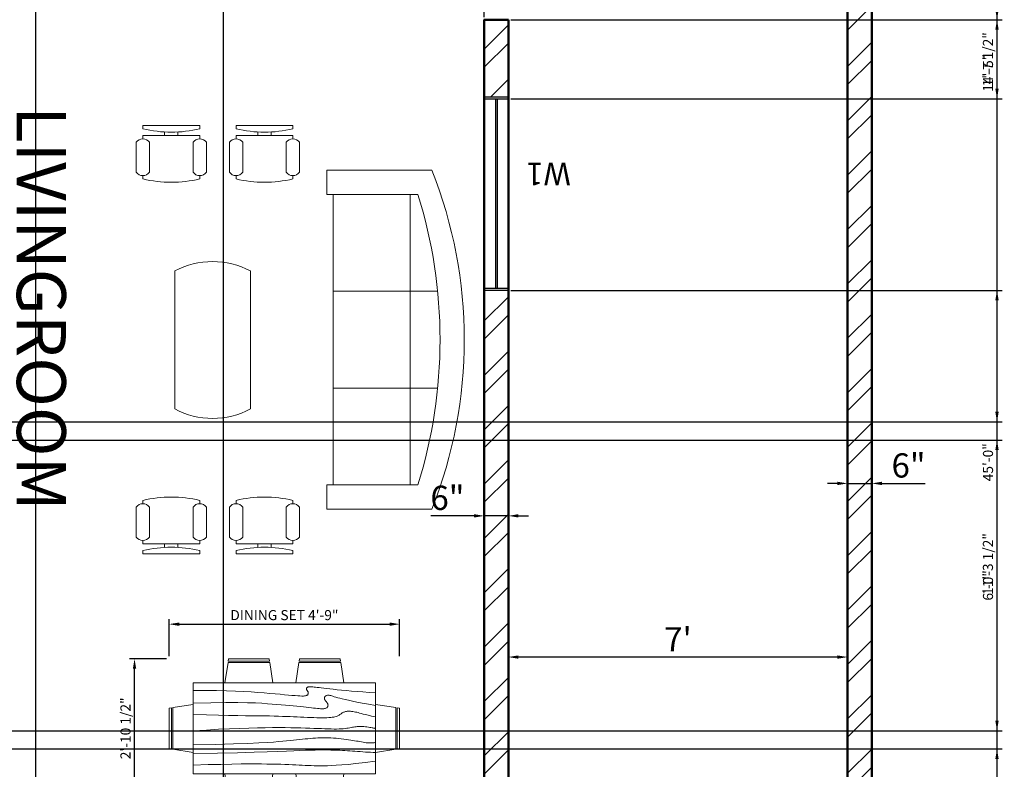
# Model space of a CAD drawing. Units: inches. Extents: x 244 to 2800, y 1060 to 1700.
# Tile 10 of 13: x 1781 to 2025, y 1287 to 1473. Entities that reach past the tile are written whole.
import ezdxf

# ---------------------------------------------------------------- set-up
doc = ezdxf.new("R2010")
doc.units = ezdxf.units.IN
for name, color, linetype, lineweight in [('A-ANNO-DIMS', 2, 'Continuous', 18), ('A-ANNO-TEXT', 1, 'Continuous', 18), ('A-FURN', 9, 'Continuous', 18), ('A-GLAZ', 3, 'Continuous', 25), ('A-WALL', 7, 'Continuous', 50), ('A-WALL-PATT', 8, 'Continuous', 13)]:
    doc.layers.add(name, color=color, linetype=linetype, lineweight=lineweight)
doc.styles.get("Standard").update_dxf_attribs({"font": 'arial.ttf'})
doc.dimstyles.new('ISO-25', dxfattribs={"dimtxt": 2.5, "dimasz": 2.5, "dimexe": 1.25, "dimexo": 0.625, "dimtad": 1, "dimlunit": 4, "dimtxsty": 'Standard', "dimcen": 2.5, "dimadec": 0, "dimazin": 0, "dimtfac": 1, "dimtmove": 0, "dimatfit": 3, "dimfxl": 1, "dimarcsym": 0})

# ---------------------------------------------------------------- blocks, each defined once
blk = doc.blocks.new('Chair - Desk')
for p, q in [((-8.5, 0), (-8.5, -1)), ((-8.5, 0), (8.5, 0)), ((8.5, 0), (8.5, -1)), ((-2, -3), (-2, -1.9355)), ((2, -1.9576), (2, -3)), ((-10.5, -5), (-10.5, -14)), ((-8.5, -3), (-8.5, -4)), ((-8.5, -3), (8.5, -3)), ((-6.5, -14), (-6.5, -5)), ((6.5, -5), (6.5, -14)), ((8.5, -3), (8.5, -4)), ((10.5, -14), (10.5, -5)), ((-8.5, -15), (-8.5, -16)), ((8.5, -15), (8.5, -16))]:
    blk.add_line(p, q)
for centre, radius, start, end in [((0, 34.625), 36.625, 256.5803, 283.4197), ((-8.5, -6.5), 2.5, 36.8699, 143.1301), ((8.5, -6.5), 2.5, 36.8699, 143.1301), ((-8.5, -12.5), 2.5, 216.8699, 323.1301), ((8.5, -12.5), 2.5, 216.8699, 323.1301), ((0, 19.625), 36.625, 256.5803, 283.4197)]:
    blk.add_arc(centre, radius, start, end)
blk = doc.blocks.new('Dining Set - 36 x 72 in.')
for p, q in [((-22, 27.5), (-22.1562, 26.50042)), ((-22, 27.5), (-6, 27.5)), ((-5.8437, 26.49966), (-6, 27.5)), ((6, 27.5), (5.8438, 26.50042)), ((6, 27.5), (22, 27.5)), ((22.1563, 26.49966), (22, 27.5)), ((-22.2343, 26.00059), (-23.4847, 17.99762)), ((-22.2304, 26), (-5.7608, 26)), ((-5.8416, 26.5), (-22.1534, 26.5)), ((-4.5152, 17.99762), (-5.7655, 25.99926)), ((5.7657, 26.00059), (4.5153, 17.99762)), ((5.7696, 26), (22.2392, 26)), ((22.1584, 26.5), (5.8466, 26.5)), ((23.4848, 17.99762), (22.2345, 25.99926)), ((36, 18), (-36, 18)), ((-36, 18), (-36, -18)), ((36, -18), (36, 18)), ((-45.5, 8), (-44.5004, 8.15617)), ((-45.5, 8), (-45.5, -8)), ((-44.5, -8.15843), (-44.5, 8.15338)), ((-44.0006, 8.23428), (-35.9976, 9.48474)), ((-44, 8.23041), (-44, -8.23915)), ((44.0006, 8.23428), (35.9976, 9.48474)), ((44, 8.23041), (44, -8.23915)), ((44.5, -8.15843), (44.5, 8.15338)), ((45.5, 8), (44.5005, 8.15617)), ((45.5, 8), (45.5, -8)), ((-44.4997, -8.15631), (-45.5, -8)), ((-35.9976, -9.48476), (-43.9993, -8.2345)), ((35.9976, -9.48476), (43.9993, -8.2345)), ((44.4997, -8.15631), (45.5, -8)), ((-36, -18), (36, -18)), ((-22.2343, -26.0006), (-23.4847, -17.99762)), ((-4.5152, -17.99762), (-5.7655, -25.99928)), ((5.7657, -26.0006), (4.5153, -17.99762)), ((23.4848, -17.99762), (22.2345, -25.99928)), ((-22.2304, -26), (-5.7608, -26)), ((-22, -27.5), (-22.1562, -26.50044)), ((-5.8416, -26.5), (-22.1534, -26.5)), ((-5.8437, -26.49967), (-6, -27.5)), ((5.7696, -26), (22.2392, -26)), ((6, -27.5), (5.8438, -26.50044)), ((22.1584, -26.5), (5.8466, -26.5)), ((22.1563, -26.49967), (22, -27.5)), ((-22, -27.5), (-6, -27.5)), ((6, -27.5), (22, -27.5))]:
    blk.add_line(p, q)
for points in [[(-36, 15), (-31.1772, 14.97754), (-26.8079, 14.91406), (-22.8538, 14.81543), (-19.276, 14.6875), (-16.0362, 14.53613), (-13.0957, 14.36718), (-10.4159, 14.18652), (-7.9583, 14), (-5.6904, 13.81315), (-3.6035, 13.63021), (-1.6954, 13.45508), (0.0365, 13.29166), (1.5945, 13.14388), (2.9811, 13.01562), (4.1988, 12.9108), (5.25, 12.83333), (6.1393, 12.78613), (6.8802, 12.76823), (7.4883, 12.77767), (7.9792, 12.8125), (8.3685, 12.87077), (8.6719, 12.95052), (8.9049, 13.0498), (9.0833, 13.16666), (9.2205, 13.29899), (9.3216, 13.44401), (9.3895, 13.59879), (9.4271, 13.76041), (9.4373, 13.92594), (9.4232, 14.09245), (9.3875, 14.257), (9.3333, 14.41666), (9.2638, 14.56917), (9.1836, 14.71484), (9.0975, 14.85465), (9.0104, 14.98958), (8.9272, 15.1206), (8.8529, 15.2487), (8.7922, 15.37483), (8.75, 15.5), (8.7305, 15.62467), (8.7344, 15.74739), (8.7617, 15.86621), (8.8125, 15.97916), (8.8867, 16.08431), (8.9844, 16.17968), (9.1055, 16.26334), (9.25, 16.33333), (9.4189, 16.38802), (9.6172, 16.42708), (9.8506, 16.45052), (10.125, 16.45833), (10.4463, 16.45052), (10.8203, 16.42708), (11.2529, 16.38802), (11.75, 16.33333), (12.3184, 16.26318), (12.9694, 16.17838), (13.7151, 16.07991), (14.5677, 15.96875), (15.5395, 15.84586), (16.6426, 15.71224), (17.8893, 15.56884), (19.2917, 15.41666), (20.859, 15.25667), (22.5879, 15.08984), (24.4721, 14.91715), (26.5052, 14.73958), (28.6809, 14.5581), (30.9929, 14.3737), (33.4347, 14.18733), (36, 14)], [(-36, 10), (-28.9766, 10.14274), (-23.1725, 10.20442), (-18.4241, 10.19775), (-14.5677, 10.13541), (-11.4399, 10.03011), (-8.877, 9.89453), (-6.7154, 9.74137), (-4.7917, 9.58333), (-2.9698, 9.43082), (-1.2246, 9.28515), (0.4415, 9.14534), (2.026, 9.01041), (3.5266, 8.87939), (4.9408, 8.7513), (6.266, 8.62516), (7.5, 8.5), (8.6411, 8.37549), (9.6914, 8.2539), (10.6538, 8.13818), (11.5312, 8.03125), (12.3267, 7.93603), (13.043, 7.85547), (13.6831, 7.79248), (14.25, 7.75), (14.7471, 7.7303), (15.1797, 7.73307), (15.5537, 7.75732), (15.875, 7.80208), (16.1494, 7.86637), (16.3828, 7.94922), (16.5811, 8.04964), (16.75, 8.16666), (16.8944, 8.29915), (17.0143, 8.44531), (17.1089, 8.60319), (17.1771, 8.77083), (17.218, 8.94629), (17.2305, 9.1276), (17.2137, 9.31282), (17.1667, 9.5), (17.0895, 9.6875), (16.987, 9.875), (16.8649, 10.0625), (16.7292, 10.25), (16.5856, 10.4375), (16.4401, 10.625), (16.2985, 10.8125), (16.1667, 11), (16.05, 11.18733), (15.9518, 11.3737), (15.8752, 11.5581), (15.8229, 11.73958), (15.798, 11.91715), (15.8034, 12.08984), (15.842, 12.25667), (15.9167, 12.41666), (16.0295, 12.56836), (16.1784, 12.70833), (16.3605, 12.83268), (16.5729, 12.9375), (16.8127, 13.01888), (17.0768, 13.07291), (17.3625, 13.0957), (17.6667, 13.08333), (17.9894, 13.03312), (18.3418, 12.94726), (18.7382, 12.82918), (19.1927, 12.68229), (19.7195, 12.51001), (20.3327, 12.31575), (21.0465, 12.10294), (21.875, 11.875), (22.8357, 11.63354), (23.959, 11.37304), (25.2786, 11.08618), (26.8282, 10.76562), (28.6414, 10.40405), (30.752, 9.99414), (33.1936, 9.52856), (36, 9)], [(-36, 5.5), (-30.7157, 5.3348), (-26.069, 5.20963), (-21.9946, 5.11767), (-18.4271, 5.05208), (-15.3009, 5.00602), (-12.5508, 4.97265), (-10.1112, 4.94515), (-7.9167, 4.91666), (-5.909, 4.88167), (-4.0586, 4.83984), (-2.3429, 4.79215), (-0.7396, 4.73958), (0.7739, 4.6831), (2.22, 4.6237), (3.6213, 4.56233), (5, 4.5), (6.373, 4.43782), (7.7344, 4.3776), (9.0723, 4.32129), (10.375, 4.27083), (11.6309, 4.22819), (12.8281, 4.19531), (13.9551, 4.17415), (15, 4.16666), (15.954, 4.17448), (16.819, 4.19791), (17.6001, 4.23698), (18.3021, 4.29166), (18.9299, 4.36198), (19.4883, 4.44791), (19.9823, 4.54948), (20.4167, 4.66666), (20.7969, 4.79899), (21.1302, 4.94401), (21.4245, 5.09879), (21.6875, 5.26041), (21.9271, 5.42594), (22.1511, 5.59245), (22.3672, 5.757), (22.5834, 5.91666), (22.8065, 6.06868), (23.0404, 6.21093), (23.2879, 6.34147), (23.5521, 6.45833), (23.8358, 6.55957), (24.142, 6.64323), (24.4735, 6.70735), (24.8334, 6.75), (25.2235, 6.76969), (25.642, 6.76692), (26.0858, 6.74267), (26.5521, 6.69791), (27.0379, 6.63362), (27.5404, 6.55078), (28.0565, 6.45036), (28.5834, 6.33333), (29.1242, 6.19987), (29.7071, 6.04687), (30.3661, 5.87044), (31.1354, 5.66666), (32.0493, 5.43164), (33.142, 5.16146), (34.4475, 4.85221), (36, 4.5)], [(-36, -1), (-30.7915, -0.6591), (-26.0195, -0.38216), (-21.6519, -0.16284), (-17.6563, 0.00521), (-14.0005, 0.12833), (-10.6523, 0.21289), (-7.5796, 0.26522), (-4.75, 0.29166), (-2.134, 0.29793), (0.2878, 0.28711), (2.5317, 0.26163), (4.6146, 0.22396), (6.5529, 0.17651), (8.3633, 0.12174), (10.0623, 0.06209), (11.6667, 0), (13.1899, -0.06201), (14.6341, -0.1211), (15.9982, -0.17432), (17.2813, -0.21875), (18.4823, -0.25147), (19.6003, -0.26953), (20.6343, -0.27002), (21.5834, -0.25), (22.4481, -0.20768), (23.2357, -0.14584), (23.9549, -0.06836), (24.6146, 0.02083), (25.2235, 0.11784), (25.7904, 0.21875), (26.3241, 0.31966), (26.8334, 0.41666), (27.3265, 0.50618), (27.8099, 0.58593), (28.2894, 0.65397), (28.7709, 0.70833), (29.2601, 0.74707), (29.763, 0.76823), (30.2855, 0.76985), (30.8334, 0.75), (31.4088, 0.70784), (31.9994, 0.64713), (32.589, 0.57275), (33.1615, 0.48958), (33.7008, 0.4025), (34.1908, 0.3164), (34.6153, 0.23616), (34.9584, 0.16666), (35.2099, 0.11165), (35.3848, 0.07031), (35.504, 0.04069), (35.5886, 0.02083), (35.6594, 0.00879), (35.7377, 0.0026), (35.8442, 0.00032), (36, 0)], [(-36, -6.5), (-27.1843, -6.31267), (-20.084, -6.1263), (-14.469, -5.9419), (-10.1094, -5.76042), (-6.7752, -5.58285), (-4.2363, -5.41016), (-2.2629, -5.24333), (-0.625, -5.08334), (0.8708, -4.93099), (2.2715, -4.78646), (3.5872, -4.64974), (4.8281, -4.52084), (6.0046, -4.39974), (7.127, -4.28646), (8.2053, -4.18099), (9.25, -4.08334), (10.2705, -3.99382), (11.2734, -3.91407), (12.2647, -3.84603), (13.25, -3.79167), (14.2354, -3.75293), (15.2266, -3.73177), (16.2295, -3.73015), (17.25, -3.75), (18.2912, -3.79248), (19.3451, -3.85547), (20.4009, -3.93604), (21.4479, -4.03125), (22.4754, -4.13819), (23.4727, -4.25391), (24.4289, -4.37549), (25.3334, -4.5), (26.1785, -4.62492), (26.9694, -4.74935), (27.7145, -4.87281), (28.4219, -4.99479), (29.1, -5.11483), (29.7572, -5.23242), (30.4016, -5.34709), (31.0417, -5.45834), (31.6837, -5.56437), (32.3262, -5.65821), (32.9658, -5.73153), (33.599, -5.77604), (34.2224, -5.78345), (34.8327, -5.74545), (35.4264, -5.65373), (36, -5.5)], [(-36, -10), (-26.4022, -9.81299), (-18.4675, -9.62891), (-11.9839, -9.45069), (-6.7396, -9.28125), (-2.5226, -9.12354), (0.8789, -8.98047), (3.6769, -8.85498), (6.0833, -8.75), (8.2767, -8.66765), (10.3021, -8.60677), (12.1712, -8.56543), (13.8958, -8.54167), (15.4876, -8.53353), (16.9583, -8.53907), (18.3197, -8.55632), (19.5834, -8.58334), (20.7616, -8.61841), (21.8685, -8.66081), (22.9188, -8.71004), (23.9271, -8.76563), (24.9081, -8.82707), (25.8763, -8.89388), (26.8465, -8.96558), (27.8334, -9.04167), (28.8474, -9.12118), (29.8828, -9.20117), (30.93, -9.27824), (31.9792, -9.34896), (33.0205, -9.40991), (34.0443, -9.45768), (35.0407, -9.48885), (36, -9.5)], [(-36, -14.5), (-30.0881, -14.33513), (-25.0332, -14.21224), (-20.7312, -14.12647), (-17.0781, -14.07292), (-13.97, -14.04671), (-11.3027, -14.04297), (-8.9724, -14.05681), (-6.875, -14.08334), (-4.9224, -14.11833), (-3.0905, -14.16016), (-1.3709, -14.20785), (0.2448, -14.26042), (1.7647, -14.3169), (3.1973, -14.3763), (4.5507, -14.43767), (5.8333, -14.5), (7.0554, -14.5621), (8.235, -14.62175), (9.3922, -14.67652), (10.5469, -14.72396), (11.7192, -14.76164), (12.929, -14.78711), (14.1965, -14.79794), (15.5417, -14.79167), (16.9933, -14.76424), (18.6152, -14.70508), (20.4804, -14.60197), (22.6615, -14.44271), (25.2312, -14.21509), (28.2624, -13.9069), (31.8277, -13.50594), (36, -13)]]:
    blk.add_lwpolyline(points)
blk = doc.blocks.new('Sofa - Roundback 7 ft.')
for p, q in [((-12.00002, -32.4421), (-12.00003, -6.5971)), ((11.99997, -32.4421), (11.99998, -6.5971)), ((-36.000027, -34), (-36.000027, -11.4696)), ((35.99998, -34), (35.99998, -11.4696)), ((-35.999844, -13.3819), (35.9998, -13.3819)), ((-36.000027, -32.4421), (35.99998, -32.4421))]:
    blk.add_line(p, q)
for points in [[(-36.000027, -34), (-42.000027, -34), (-42.000027, -8)], [(41.99998, -8), (41.99998, -34), (35.99998, -34)]]:
    blk.add_lwpolyline(points)
for centre, radius, start, end in [((0, -114.25), 114.25, 68.43141, 111.5686), ((-0.00001, -127.1968), 121.1968, 72.72033, 107.2797)]:
    blk.add_arc(centre, radius, start, end)
blk = doc.blocks.new('*D25')
at = {"layer": 'A-ANNO-DIMS', "color": 0, "lineweight": -2, "transparency": 16777216}
for p, q in [((1902.4, 1299.07), (1902.4, 1315.98)), ((1983.9, 1314.73), (1904.9, 1314.73)), ((1986.4, 1299.07), (1986.4, 1315.98))]:
    blk.add_line(p, q, dxfattribs=at)
at = {"layer": 'A-ANNO-DIMS', "color": 0, "transparency": 16777216}
for points in [[(1904.9, 1315.14), (1904.9, 1314.31), (1902.4, 1314.73)], [(1983.9, 1315.14), (1983.9, 1314.31), (1986.4, 1314.73)]]:
    blk.add_solid(points, dxfattribs=at)
at = {"layer": 'Defpoints', "color": 0, "transparency": 16777216}
for p in [(1902.4, 1314.73), (1902.4, 1298.44), (1986.4, 1298.44)]:
    blk.add_point(p, dxfattribs=at)
at = {"layer": 'A-ANNO-DIMS', "color": 0, "transparency": 16777216, "insert": (1944.4, 1318.35), "char_height": 6, "attachment_point": 5}
blk.add_mtext("7'", dxfattribs=at)
blk = doc.blocks.new('*D26')
at = {"layer": 'A-ANNO-DIMS', "color": 0, "lineweight": -2, "transparency": 16777216}
for p, q in [((1896.4, 1340.06), (1896.4, 1350.96)), ((1902.4, 1340.06), (1902.4, 1350.96)), ((1893.9, 1349.71), (1883.22, 1349.71)), ((1902.4, 1349.71), (1896.4, 1349.71)), ((1904.9, 1349.71), (1907.4, 1349.71))]:
    blk.add_line(p, q, dxfattribs=at)
at = {"layer": 'A-ANNO-DIMS', "color": 0, "transparency": 16777216}
for points in [[(1893.9, 1350.13), (1893.9, 1349.3), (1896.4, 1349.71)], [(1904.9, 1350.13), (1904.9, 1349.3), (1902.4, 1349.71)]]:
    blk.add_solid(points, dxfattribs=at)
at = {"layer": 'Defpoints', "color": 0, "transparency": 16777216}
for p in [(1896.4, 1349.71), (1896.4, 1339.43), (1902.4, 1339.43)]:
    blk.add_point(p, dxfattribs=at)
at = {"layer": 'A-ANNO-DIMS', "color": 0, "transparency": 16777216, "insert": (1887.31, 1353.4), "char_height": 6, "attachment_point": 5}
blk.add_mtext('6"', dxfattribs=at)
blk = doc.blocks.new('*D27')
at = {"layer": 'A-ANNO-DIMS', "color": 0, "lineweight": -2, "transparency": 16777216}
for p, q in [((1986.4, 1358.37), (1986.4, 1359)), ((1992.4, 1358.37), (1992.4, 1359)), ((1983.9, 1357.75), (1981.4, 1357.75)), ((1986.4, 1357.75), (1992.4, 1357.75)), ((1994.9, 1357.75), (2005.57, 1357.75))]:
    blk.add_line(p, q, dxfattribs=at)
at = {"layer": 'A-ANNO-DIMS', "color": 0, "transparency": 16777216}
for points in [[(1983.9, 1358.16), (1983.9, 1357.33), (1986.4, 1357.75)], [(1994.9, 1358.16), (1994.9, 1357.33), (1992.4, 1357.75)]]:
    blk.add_solid(points, dxfattribs=at)
at = {"layer": 'Defpoints', "color": 0, "transparency": 16777216}
for p in [(1986.4, 1357.75), (1992.4, 1357.75), (1992.4, 1357.75)]:
    blk.add_point(p, dxfattribs=at)
at = {"layer": 'A-ANNO-DIMS', "color": 0, "transparency": 16777216, "insert": (2001.49, 1361.43), "char_height": 6, "attachment_point": 5}
blk.add_mtext('6"', dxfattribs=at)
blk = doc.blocks.new('WIN-48')
for p, q in [((0, 0), (0, 47.95)), ((0, 47.95), (6, 47.95)), ((6, 47.95), (6, 0)), ((6, 0), (0, 0))]:
    blk.add_line(p, q)
blk = doc.blocks.new('*D72')
at = {"layer": 'A-ANNO-DIMS', "color": 0, "lineweight": -2, "transparency": 16777216}
for p, q in [((1818.4, 1314.94), (1818.4, 1324.13)), ((1875.48, 1314.94), (1875.48, 1324.13)), ((1820.9, 1322.88), (1872.98, 1322.88))]:
    blk.add_line(p, q, dxfattribs=at)
at = {"layer": 'A-ANNO-DIMS', "color": 0, "transparency": 16777216}
for points in [[(1820.9, 1323.29), (1820.9, 1322.46), (1818.4, 1322.88)], [(1872.98, 1323.29), (1872.98, 1322.46), (1875.48, 1322.88)]]:
    blk.add_solid(points, dxfattribs=at)
at = {"layer": 'Defpoints', "color": 0, "transparency": 16777216}
for p in [(1875.48, 1322.88), (1818.4, 1314.32), (1875.48, 1314.32)]:
    blk.add_point(p, dxfattribs=at)
at = {"layer": 'A-ANNO-DIMS', "color": 0, "transparency": 16777216, "insert": (1846.94, 1324.8), "char_height": 2.5, "attachment_point": 5}
blk.add_mtext('DINING SET 4\'-9"', dxfattribs=at)
blk = doc.blocks.new('*D73')
at = {"layer": 'A-ANNO-DIMS', "color": 0, "lineweight": -2, "transparency": 16777216}
for p, q in [((1817.77, 1314.32), (1808.58, 1314.32)), ((1809.83, 1282.32), (1809.83, 1311.82)), ((1817.77, 1279.82), (1808.58, 1279.82))]:
    blk.add_line(p, q, dxfattribs=at)
at = {"layer": 'A-ANNO-DIMS', "color": 0, "transparency": 16777216}
for points in [[(1809.42, 1311.82), (1810.25, 1311.82), (1809.83, 1314.32)], [(1809.42, 1282.32), (1810.25, 1282.32), (1809.83, 1279.82)]]:
    blk.add_solid(points, dxfattribs=at)
at = {"layer": 'Defpoints', "color": 0, "transparency": 16777216}
for p in [(1809.83, 1314.32), (1818.4, 1314.32), (1818.4, 1279.82)]:
    blk.add_point(p, dxfattribs=at)
at = {"layer": 'A-ANNO-DIMS', "color": 0, "transparency": 16777216, "insert": (1807.92, 1297.07), "char_height": 2.5, "attachment_point": 5, "rotation": 90}
blk.add_mtext('2\'-10 1/2"', dxfattribs=at)
blk = doc.blocks.new('*D75')
at = {"layer": 'A-ANNO-DIMS', "color": 0, "lineweight": -2, "transparency": 16777216}
for p, q in [((1993.02, 1632.99), (2024.65, 1632.99)), ((2023.4, 1095.49), (2023.4, 1630.49)), ((1993.02, 1092.99), (2024.65, 1092.99))]:
    blk.add_line(p, q, dxfattribs=at)
at = {"layer": 'A-ANNO-DIMS', "color": 0, "transparency": 16777216}
for points in [[(2022.98, 1630.49), (2023.81, 1630.49), (2023.4, 1632.99)], [(2022.98, 1095.49), (2023.81, 1095.49), (2023.4, 1092.99)]]:
    blk.add_solid(points, dxfattribs=at)
at = {"layer": 'Defpoints', "color": 0, "transparency": 16777216}
for p in [(1992.4, 1632.99), (2023.4, 1632.99), (1992.4, 1092.99)]:
    blk.add_point(p, dxfattribs=at)
at = {"layer": 'A-ANNO-DIMS', "color": 0, "transparency": 16777216, "insert": (2021.49, 1362.99), "char_height": 2.5, "attachment_point": 5, "rotation": 90}
blk.add_mtext('45\'-0"', dxfattribs=at)
blk = doc.blocks.new('*D85')
at = {"layer": 'A-ANNO-DIMS', "color": 0, "lineweight": -2, "transparency": 16777216}
for p, q in [((1537.02, 1291.99), (2024.65, 1291.99)), ((2023.4, 1119.49), (2023.4, 1289.49)), ((1537.02, 1116.99), (2024.65, 1116.99))]:
    blk.add_line(p, q, dxfattribs=at)
at = {"layer": 'A-ANNO-DIMS', "color": 0, "transparency": 16777216}
for points in [[(2022.98, 1289.49), (2023.81, 1289.49), (2023.4, 1291.99)], [(2022.98, 1119.49), (2023.81, 1119.49), (2023.4, 1116.99)]]:
    blk.add_solid(points, dxfattribs=at)
at = {"layer": 'Defpoints', "color": 0, "transparency": 16777216}
for p in [(1536.4, 1291.99), (2023.4, 1291.99), (1536.4, 1116.99)]:
    blk.add_point(p, dxfattribs=at)
at = {"layer": 'A-ANNO-DIMS', "color": 0, "transparency": 16777216, "insert": (2021.52, 1204.49), "char_height": 2.5, "attachment_point": 5, "rotation": 90}
blk.add_mtext('14\'-7"', dxfattribs=at)
blk = doc.blocks.new('*D86')
at = {"layer": 'A-ANNO-DIMS', "color": 0, "lineweight": -2, "transparency": 16777216}
for p, q in [((1537.02, 1368.49), (2024.65, 1368.49)), ((2023.4, 1298.99), (2023.4, 1365.99)), ((1537.02, 1296.49), (2024.65, 1296.49))]:
    blk.add_line(p, q, dxfattribs=at)
at = {"layer": 'A-ANNO-DIMS', "color": 0, "transparency": 16777216}
for points in [[(2022.98, 1365.99), (2023.81, 1365.99), (2023.4, 1368.49)], [(2022.98, 1298.99), (2023.81, 1298.99), (2023.4, 1296.49)]]:
    blk.add_solid(points, dxfattribs=at)
at = {"layer": 'Defpoints', "color": 0, "transparency": 16777216}
for p in [(1536.4, 1368.49), (2023.4, 1368.49), (1536.4, 1296.49)]:
    blk.add_point(p, dxfattribs=at)
at = {"layer": 'A-ANNO-DIMS', "color": 0, "transparency": 16777216, "insert": (2021.49, 1332.49), "char_height": 2.5, "attachment_point": 5, "rotation": 90}
blk.add_mtext('6\'-0"', dxfattribs=at)
blk = doc.blocks.new('*D87')
at = {"layer": 'A-ANNO-DIMS', "color": 0, "lineweight": -2, "transparency": 16777216}
for p, q in [((1537.02, 1545.99), (2024.65, 1545.99)), ((2023.4, 1375.49), (2023.4, 1543.49)), ((1537.02, 1372.99), (2024.65, 1372.99))]:
    blk.add_line(p, q, dxfattribs=at)
at = {"layer": 'A-ANNO-DIMS', "color": 0, "transparency": 16777216}
for points in [[(2022.98, 1543.49), (2023.81, 1543.49), (2023.4, 1545.99)], [(2022.98, 1375.49), (2023.81, 1375.49), (2023.4, 1372.99)]]:
    blk.add_solid(points, dxfattribs=at)
at = {"layer": 'Defpoints', "color": 0, "transparency": 16777216}
for p in [(1536.4, 1545.99), (2023.4, 1545.99), (1536.4, 1372.99)]:
    blk.add_point(p, dxfattribs=at)
at = {"layer": 'A-ANNO-DIMS', "color": 0, "transparency": 16777216, "insert": (2021.49, 1459.49), "char_height": 2.5, "attachment_point": 5, "rotation": 90}
blk.add_mtext('14\'-5"', dxfattribs=at)
blk = doc.blocks.new('*D90')
at = {"layer": 'A-ANNO-DIMS', "color": 0, "lineweight": -2, "transparency": 16777216}
for p, q in [((1708.9, 1491.26), (1708.9, 1665.24)), ((1896.4, 1473.26), (1896.4, 1665.24)), ((1711.4, 1663.99), (1893.9, 1663.99))]:
    blk.add_line(p, q, dxfattribs=at)
at = {"layer": 'A-ANNO-DIMS', "color": 0, "transparency": 16777216}
for points in [[(1711.4, 1664.4), (1711.4, 1663.57), (1708.9, 1663.99)], [(1893.9, 1664.4), (1893.9, 1663.57), (1896.4, 1663.99)]]:
    blk.add_solid(points, dxfattribs=at)
at = {"layer": 'Defpoints', "color": 0, "transparency": 16777216}
for p in [(1896.4, 1663.99), (1708.9, 1490.64), (1896.4, 1472.64)]:
    blk.add_point(p, dxfattribs=at)
at = {"layer": 'A-ANNO-DIMS', "color": 0, "transparency": 16777216, "insert": (1802.65, 1665.9), "char_height": 2.5, "attachment_point": 5}
blk.add_mtext('15\'-7 1/2"', dxfattribs=at)
blk = doc.blocks.new('*D99')
at = {"layer": 'A-ANNO-DIMS', "color": 0, "lineweight": -2, "transparency": 16777216}
for p, q in [((1903.02, 1472.64), (2024.65, 1472.64)), ((2023.4, 1455.53), (2023.4, 1470.14)), ((1903.02, 1453.03), (2024.65, 1453.03))]:
    blk.add_line(p, q, dxfattribs=at)
at = {"layer": 'A-ANNO-DIMS', "color": 0, "transparency": 16777216}
for points in [[(2022.98, 1470.14), (2023.81, 1470.14), (2023.4, 1472.64)], [(2022.98, 1455.53), (2023.81, 1455.53), (2023.4, 1453.03)]]:
    blk.add_solid(points, dxfattribs=at)
at = {"layer": 'Defpoints', "color": 0, "transparency": 16777216}
for p in [(1902.4, 1472.64), (2023.4, 1472.64), (1902.4, 1453.03)]:
    blk.add_point(p, dxfattribs=at)
at = {"layer": 'A-ANNO-DIMS', "color": 0, "transparency": 16777216, "insert": (2021.48, 1462.83), "char_height": 2.5, "attachment_point": 5, "rotation": 90}
blk.add_mtext('1\'-7 1/2"', dxfattribs=at)
blk = doc.blocks.new('*D100')
at = {"layer": 'A-ANNO-DIMS', "color": 0, "lineweight": -2, "transparency": 16777216}
for p, q in [((1903.02, 1532.64), (2024.65, 1532.64)), ((2023.4, 1475.14), (2023.4, 1530.14)), ((1903.02, 1472.64), (2024.65, 1472.64))]:
    blk.add_line(p, q, dxfattribs=at)
at = {"layer": 'A-ANNO-DIMS', "color": 0, "transparency": 16777216}
for points in [[(2022.98, 1530.14), (2023.81, 1530.14), (2023.4, 1532.64)], [(2022.98, 1475.14), (2023.81, 1475.14), (2023.4, 1472.64)]]:
    blk.add_solid(points, dxfattribs=at)
at = {"layer": 'Defpoints', "color": 0, "transparency": 16777216}
for p in [(1902.4, 1532.64), (2023.4, 1532.64), (1902.4, 1472.64)]:
    blk.add_point(p, dxfattribs=at)
at = {"layer": 'A-ANNO-DIMS', "color": 0, "transparency": 16777216, "insert": (2021.49, 1502.64), "char_height": 2.5, "attachment_point": 5, "rotation": 90}
blk.add_mtext('5\'-0"', dxfattribs=at)
blk = doc.blocks.new('*D102')
at = {"layer": 'A-ANNO-DIMS', "color": 0, "lineweight": -2, "transparency": 16777216}
for p, q in [((1903.02, 1405.58), (2024.65, 1405.58)), ((2023.4, 1272.49), (2023.4, 1403.08)), ((1903.02, 1269.99), (2024.65, 1269.99))]:
    blk.add_line(p, q, dxfattribs=at)
at = {"layer": 'A-ANNO-DIMS', "color": 0, "transparency": 16777216}
for points in [[(2022.98, 1403.08), (2023.81, 1403.08), (2023.4, 1405.58)], [(2022.98, 1272.49), (2023.81, 1272.49), (2023.4, 1269.99)]]:
    blk.add_solid(points, dxfattribs=at)
at = {"layer": 'Defpoints', "color": 0, "transparency": 16777216}
for p in [(1902.4, 1405.58), (2023.4, 1405.58), (1902.4, 1269.99)]:
    blk.add_point(p, dxfattribs=at)
at = {"layer": 'A-ANNO-DIMS', "color": 0, "transparency": 16777216, "insert": (2021.48, 1337.78), "char_height": 2.5, "attachment_point": 5, "rotation": 90}
blk.add_mtext('11\'-3 1/2"', dxfattribs=at)
blk = doc.blocks.new('*D104')
at = {"layer": 'A-ANNO-DIMS', "color": 0, "lineweight": -2, "transparency": 16777216}
for p, q in [((1785.4, 1201.61), (1785.4, 1665.24)), ((1831.9, 1206.11), (1831.9, 1665.24)), ((1787.9, 1663.99), (1829.4, 1663.99))]:
    blk.add_line(p, q, dxfattribs=at)
at = {"layer": 'A-ANNO-DIMS', "color": 0, "transparency": 16777216}
for points in [[(1787.9, 1664.4), (1787.9, 1663.57), (1785.4, 1663.99)], [(1829.4, 1664.4), (1829.4, 1663.57), (1831.9, 1663.99)]]:
    blk.add_solid(points, dxfattribs=at)
at = {"layer": 'Defpoints', "color": 0, "transparency": 16777216}
for p in [(1831.9, 1663.99), (1831.9, 1205.49), (1785.4, 1200.99)]:
    blk.add_point(p, dxfattribs=at)
at = {"layer": 'A-ANNO-DIMS', "color": 0, "transparency": 16777216, "insert": (1808.65, 1665.9), "char_height": 2.5, "attachment_point": 5}
blk.add_mtext('3\'-10 1/2"', dxfattribs=at)

msp = doc.modelspace()

# ---------------------------------------------------------------- hatches: boundary and pattern name
at = {"layer": 'A-WALL-PATT'}
h = msp.add_hatch(dxfattribs=at)
h.set_pattern_fill('ANSI32', color=256)
h.paths.add_polyline_path([(1992.396, 1092.986), (1992.396, 1632.986), (1512.396, 1632.986), (1512.396, 1092.986)])
h.paths.add_polyline_path([(1518.396, 1098.986), (1518.396, 1626.986), (1986.396, 1626.986), (1986.396, 1098.986), (1902.396, 1098.986)], flags=16)
h.paths.add_polyline_path([(1795.896, 1110.986), (1530.396, 1110.986), (1530.396, 1551.986), (1521.7, 1551.986), (1521.7, 1623.986), (1605.7, 1623.986), (1605.7, 1551.986), (1781.396, 1551.986), (1781.396, 1545.986), (1708.896, 1545.986), (1708.896, 1532.64), (1704.396, 1532.64), (1704.396, 1545.986), (1536.396, 1545.986), (1536.396, 1372.986), (1671.396, 1372.986), (1671.396, 1368.486), (1621.896, 1368.486), (1621.896, 1296.486), (1704.396, 1296.486), (1704.396, 1368.486), (1701.396, 1368.486), (1701.396, 1372.986), (1704.396, 1372.986), (1704.396, 1490.64), (1708.896, 1490.64), (1708.896, 1288.986), (1704.396, 1288.986), (1704.396, 1291.986), (1569.396, 1291.986), (1569.396, 1296.486), (1618.896, 1296.486), (1618.896, 1368.486), (1536.396, 1368.486), (1536.396, 1296.486), (1539.396, 1296.486), (1539.396, 1291.986), (1536.396, 1291.986), (1536.396, 1116.986), (1704.396, 1116.986), (1704.396, 1246.986), (1708.896, 1246.986), (1708.896, 1116.986), (1744.896, 1116.986), (1744.896, 1260.986), (1780.896, 1260.986), (1785.396, 1260.986), (1785.396, 1205.486), (1831.896, 1205.486), (1831.896, 1217.486), (1836.396, 1217.486), (1836.396, 1205.486), (1896.396, 1205.486), (1896.396, 1265.486), (1836.396, 1265.486), (1836.396, 1253.486), (1831.896, 1253.486), (1831.896, 1269.986), (1896.396, 1269.986), (1896.396, 1472.64), (1902.396, 1472.64), (1902.396, 1242.986), (1938.396, 1242.986), (1938.396, 1134.986), (1950.396, 1134.986), (1950.396, 1242.986), (1986.396, 1242.986), (1986.396, 1134.986), (1902.396, 1134.986), (1902.396, 1110.986), (1831.896, 1110.986), (1831.896, 1116.986), (1896.396, 1116.986), (1896.396, 1200.986), (1785.396, 1200.986), (1785.396, 1116.986), (1795.896, 1116.986)], flags=0)
h.paths.add_polyline_path([(1780.896, 1116.986), (1744.896, 1116.986), (1744.896, 1260.986), (1780.896, 1260.986)], flags=0)
h.paths.add_polyline_path([(1863.351, 1110.986), (1863.351, 1116.986), (1887.296, 1116.986), (1887.296, 1110.986)], flags=0)
h.paths.add_polyline_path([(1863.851, 1114.186), (1886.796, 1114.186), (1886.796, 1113.786), (1863.851, 1113.786)], flags=0)
h.paths.add_polyline_path([(1896.396, 1174.102), (1896.396, 1198.047), (1902.396, 1198.047), (1902.396, 1174.102)], flags=0)
h.paths.add_polyline_path([(1902.396, 1174.602), (1899.196, 1174.602), (1899.196, 1197.547), (1902.396, 1197.547)], flags=0)
h.paths.add_polyline_path([(1692.519, 1110.986), (1656.574, 1110.986), (1656.574, 1116.986), (1692.519, 1116.986)], flags=0)
h.paths.add_polyline_path([(1819.776, 1376.187), (1819.776, 1410.382, -0.249194), (1838.546, 1410.382), (1838.546, 1376.187, -0.249194)], flags=0)
h.paths.add_polyline_path([(1536.396, 1250.972), (1530.396, 1250.972), (1530.396, 1286.917), (1536.396, 1286.917)], flags=0)
h.paths.add_polyline_path([(1896.396, 1405.581), (1896.396, 1453.526), (1902.396, 1453.526), (1902.396, 1405.581)], flags=0)
h.paths.add_polyline_path([(1536.396, 1322.935), (1530.396, 1322.935), (1530.396, 1346.88), (1536.396, 1346.88)], flags=0)
h.paths.add_polyline_path([(1533.196, 1323.435), (1533.196, 1346.38), (1533.596, 1346.38), (1533.596, 1323.435)], flags=0)
h.paths.add_polyline_path([(1896.396, 1545.986), (1841.396, 1545.986), (1841.396, 1551.986), (1902.396, 1551.986), (1902.396, 1532.64), (1896.396, 1532.64)], flags=0)
h.paths.add_polyline_path([(1756.808, 1545.986), (1732.863, 1545.986), (1732.863, 1551.986), (1756.808, 1551.986)], flags=0)
h.paths.add_polyline_path([(1756.308, 1548.786), (1733.363, 1548.786), (1733.363, 1551.986), (1756.308, 1551.986)], flags=0)
h.paths.add_polyline_path([(1673.743, 1545.986), (1637.798, 1545.986), (1637.798, 1551.986), (1673.743, 1551.986)], flags=0)
h.paths.add_polyline_path([(1536.396, 1503.969), (1530.396, 1503.969), (1530.396, 1539.914), (1536.396, 1539.914)], flags=0)
h.paths.add_polyline_path([(1896.341, 1192.868), (1881.737, 1192.868), (1881.737, 1181.273), (1896.341, 1181.273)], flags=8)
h.paths.add_polyline_path([(1882.893, 1112.542), (1868.29, 1112.542), (1868.29, 1100.947), (1882.893, 1100.947)], flags=8)
h.paths.add_polyline_path([(1531.898, 1340.208), (1517.295, 1340.208), (1517.295, 1328.613), (1531.898, 1328.613)], flags=24)
h.paths.add_polyline_path([(1662.207, 1564.332), (1647.603, 1564.332), (1647.603, 1552.737), (1662.207, 1552.737)], flags=8)
h.paths.add_polyline_path([(1750.605, 1565.018), (1736.001, 1565.018), (1736.001, 1553.424), (1750.605, 1553.424)], flags=8)
h.paths.add_polyline_path([(1919.351, 1440.326), (1904.748, 1440.326), (1904.748, 1428.731), (1919.351, 1428.731)], flags=8)
h.paths.add_polyline_path([(1827.662, 1149.994), (1797.512, 1149.994), (1797.512, 1122.813), (1827.662, 1122.813)], flags=8)
h.paths.add_polyline_path([(1826.683, 1247.85), (1796.533, 1247.85), (1796.533, 1220.668), (1826.683, 1220.668)], flags=8)
h.paths.add_polyline_path([(1713.043, 1285.137), (1682.893, 1285.137), (1682.893, 1257.956), (1713.043, 1257.956)], flags=8)
h.paths.add_polyline_path([(1567.301, 1310.129), (1537.151, 1310.129), (1537.151, 1282.948), (1567.301, 1282.948)], flags=8)
h.paths.add_polyline_path([(1699.655, 1386.046), (1669.505, 1386.046), (1669.505, 1358.865), (1699.655, 1358.865)], flags=8)
h.paths.add_polyline_path([(1716.254, 1527.375), (1686.103, 1527.375), (1686.103, 1500.194), (1716.254, 1500.194)], flags=8)
h.paths.add_polyline_path([(1822.088, 1577.207), (1791.938, 1577.207), (1791.938, 1550.026), (1822.088, 1550.026)], flags=8)
h.paths.add_polyline_path([(1931.716, 1518.23), (1901.565, 1518.23), (1901.565, 1491.049), (1931.716, 1491.049)], flags=8)
h.paths.add_polyline_path([(1636.272, 1573.477), (1636.272, 1615.869), (1613.819, 1615.869), (1613.819, 1573.477)], flags=8)
h.paths.add_polyline_path([(1968.141, 1266.003), (1911.144, 1266.003), (1911.144, 1252.05), (1968.141, 1252.05)], flags=8)
h.paths.add_polyline_path([(1783.26, 1275.202), (1745.711, 1275.202), (1745.711, 1261.249), (1783.26, 1261.249)], flags=8)
h.paths.add_polyline_path([(1753.522, 1456.095), (1753.522, 1338.024), (1798.876, 1338.024), (1798.876, 1456.095)], flags=8)
h.paths.add_polyline_path([(1884.04, 1192.467), (1803.345, 1192.467), (1803.345, 1149.693), (1884.04, 1149.693)], flags=8)
h.paths.add_polyline_path([(1863.426, 1264.753), (1863.426, 1209.557), (1892.661, 1209.557), (1892.661, 1264.753)], flags=8)
h.paths.add_polyline_path([(1594.411, 1361.178), (1536.688, 1361.178), (1536.688, 1330.387), (1594.411, 1330.387)], flags=8)
h.paths.add_polyline_path([(1695.984, 1342.402), (1638.262, 1342.402), (1638.262, 1311.611), (1695.984, 1311.611)], flags=8)
h.paths.add_polyline_path([(1654.435, 1540.65), (1537.752, 1540.65), (1537.752, 1489.721), (1654.435, 1489.721)], flags=8)
h.paths.add_polyline_path([(1658.864, 1271.272), (1542.182, 1271.272), (1542.182, 1220.343), (1658.864, 1220.343)], flags=8)
h = msp.add_hatch(dxfattribs=at)
h.set_pattern_fill('ANSI32', color=256)
h.paths.add_polyline_path([(1902.396, 1472.64), (1896.396, 1472.64), (1896.396, 1453.526), (1902.396, 1453.526)])
h = msp.add_hatch(dxfattribs=at)
h.set_pattern_fill('ANSI32', color=256)
h.paths.add_polyline_path([(1902.396, 1405.581), (1896.396, 1405.581), (1896.396, 1269.986), (1902.396, 1269.986)])

# ---------------------------------------------------------------- linework, layer by layer
at = {"layer": 'A-FURN'}
for p, q in [((1819.776, 1376.187), (1819.776, 1410.382)), ((1819.776, 1410.382), (1819.776, 1410.382)), ((1838.546, 1410.382), (1838.546, 1410.382)), ((1838.546, 1410.382), (1838.546, 1376.187)), ((1819.776, 1376.187), (1819.776, 1376.187)), ((1838.546, 1376.187), (1838.546, 1376.187))]:
    msp.add_line(p, q, dxfattribs=at)
for centre, start, end in [((1829.161, 1392.721), 62.01446, 117.98554), ((1829.161, 1393.849), 242.01446, 297.98554)]:
    msp.add_arc(centre, 20, start, end, dxfattribs=at)
at = {"layer": 'A-GLAZ'}
for p, q in [((1896.396, 1453.026), (1902.396, 1453.026)), ((1899.196, 1453.026), (1899.196, 1406.081)), ((1899.596, 1453.026), (1899.596, 1406.081)), ((1902.396, 1406.081), (1896.396, 1406.081))]:
    msp.add_line(p, q, dxfattribs=at)
at = {"layer": 'A-WALL'}
for p, q in [((1992.396, 1092.986), (1992.396, 1632.986)), ((1986.396, 1098.986), (1986.396, 1626.986)), ((1896.317, 1472.64), (1902.396, 1472.64)), ((1896.396, 1116.986), (1896.396, 1472.64)), ((1902.396, 1098.986), (1902.396, 1472.64))]:
    msp.add_line(p, q, dxfattribs=at)

# ---------------------------------------------------------------- block references
at = {"layer": 'A-FURN'}
for name, p, xscale, yscale, zscale in [('Chair - Desk', (1818.937, 1446.432), 0.8278982100780222, 0.8278982100780222, 0.8278982100780222), ('Chair - Desk', (1842.006, 1446.432), 0.8278982100780222, 0.8278982100780222, 0.8278982100780222), ('Dining Set - 36 x 72 in.', (1846.937, 1297.066), 0.627265132509438, 0.627265132509438, 0.627265132509438)]:
    msp.add_blockref(name, p, dxfattribs=dict(at, xscale=xscale, yscale=yscale, zscale=zscale))
at = {"layer": 'A-FURN', "rotation": 270}
msp.add_blockref('Sofa - Roundback 7 ft.', (1891.48, 1393.362), dxfattribs=at)
at = {"layer": 'A-FURN', "xscale": -0.8278982100780222, "yscale": 0.8278982100780222, "zscale": 0.8278982100780222, "rotation": 180}
for p in [(1818.937, 1340.292), (1842.006, 1340.292)]:
    msp.add_blockref('Chair - Desk', p, dxfattribs=at)
at = {"layer": 'A-GLAZ'}
msp.add_blockref('WIN-48', (1896.396, 1405.581), dxfattribs=at)

# ---------------------------------------------------------------- texts
at = {"layer": 'A-ANNO-TEXT', "attachment_point": 1}
for s, width, gutter_width, insert, char_height, rotation in [('LIVINGROOM\\P15\'-7.5"X23\'-0"', 101.44398, 60.772, (1792.837, 1451.207), 12.15447, 270), ('W1', 2.91536, 28.132, (1917.849, 1431.604), 5.6265, 180)]:
    msp.add_mtext_dynamic_manual_height_columns(s, width=width, gutter_width=gutter_width, heights=[0], dxfattribs=dict(at, insert=insert, char_height=char_height, rotation=rotation))

# ---------------------------------------------------------------- dimensions: what is measured, and where the dimension line sits
at = {"layer": 'A-ANNO-DIMS'}
for base, p1, p2, override, picture, middle in [((1896.396, 1663.986), (1708.896, 1490.64), (1896.396, 1472.64), {"dimdec": 1, "dimlfac": 1, "dimrnd": 0, "dimzin": 1, "dimdsep": 46, "dimlunit": 4, "dimfrac": 2}, '*D90', (1802.646, 1665.904)), ((1831.896, 1663.986), (1785.396, 1200.986), (1831.896, 1205.486), {"dimdec": 1, "dimlfac": 1, "dimrnd": 0, "dimzin": 1, "dimdsep": 46, "dimlunit": 4, "dimfrac": 2}, '*D104', (1808.646, 1665.905)), ((1992.396, 1357.746), (1986.396, 1357.746), (1992.396, 1357.746), {"dimtxt": 6, "dimclrd": 0, "dimclre": 0, "dimclrt": 0}, '*D27', (2001.485, 1361.434)), ((1896.396, 1349.715), (1902.396, 1339.433), (1896.396, 1339.433), {"dimtxt": 6, "dimclrd": 0, "dimclre": 0, "dimclrt": 0}, '*D26', (1887.306, 1353.403)), ((1902.396, 1314.725), (1986.396, 1298.443), (1902.396, 1298.443), {"dimtxt": 6, "dimclrd": 0, "dimclre": 0, "dimclrt": 0}, '*D25', (1944.396, 1318.35))]:
    dim = msp.add_linear_dim(base=base, p1=p1, p2=p2, dimstyle='ISO-25', override=override, dxfattribs=at)
    dim.commit()
    dim.dimension.update_dxf_attribs({"geometry": picture, "text_midpoint": middle})
for base, p1, p2, override, picture, middle in [((2023.396, 1632.986), (1992.396, 1092.986), (1992.396, 1632.986), {"dimdec": 1, "dimlfac": 1, "dimrnd": 0, "dimzin": 1, "dimdsep": 46, "dimlunit": 4, "dimfrac": 2}, '*D75', (2021.494, 1362.986)), ((2023.396, 1545.986), (1536.396, 1372.986), (1536.396, 1545.986), {"dimdec": 1, "dimlfac": 1, "dimrnd": 0, "dimzin": 1, "dimdsep": 46, "dimlunit": 4, "dimfrac": 2}, '*D87', (2021.494, 1459.486)), ((2023.396, 1532.64), (1902.396, 1472.64), (1902.396, 1532.64), {"dimdec": 1, "dimlfac": 1, "dimrnd": 0, "dimzin": 1, "dimdsep": 46, "dimlunit": 4, "dimfrac": 2}, '*D100', (2021.494, 1502.64)), ((2023.396, 1472.64), (1902.396, 1453.026), (1902.396, 1472.64), {"dimdec": 1, "dimlfac": 1, "dimrnd": 0, "dimzin": 1, "dimdsep": 46, "dimlunit": 4, "dimfrac": 2}, '*D99', (2021.478, 1462.833)), ((2023.396, 1405.581), (1902.396, 1269.986), (1902.396, 1405.581), {"dimdec": 1, "dimlfac": 1, "dimrnd": 0, "dimzin": 1, "dimdsep": 46, "dimlunit": 4, "dimfrac": 2}, '*D102', (2021.477, 1337.784)), ((2023.396, 1368.486), (1536.396, 1296.486), (1536.396, 1368.486), {"dimdec": 1, "dimlfac": 1, "dimrnd": 0, "dimzin": 1, "dimdsep": 46, "dimlunit": 4, "dimfrac": 2}, '*D86', (2021.494, 1332.486)), ((1809.834, 1314.316), (1818.397, 1279.816), (1818.397, 1314.316), {"dimdec": 1, "dimrnd": 0, "dimzin": 1, "dimlunit": 4, "dimfrac": 2}, '*D73', (1807.917, 1297.066)), ((2023.396, 1291.986), (1536.396, 1116.986), (1536.396, 1291.986), {"dimdec": 1, "dimlfac": 1, "dimrnd": 0, "dimzin": 1, "dimdsep": 46, "dimlunit": 4, "dimfrac": 2}, '*D85', (2021.516, 1204.486))]:
    dim = msp.add_linear_dim(base=base, p1=p1, p2=p2, angle=90, dimstyle='ISO-25', override=override, dxfattribs=at)
    dim.commit()
    dim.dimension.update_dxf_attribs({"geometry": picture, "text_midpoint": middle})
dim = msp.add_linear_dim(base=(1875.478, 1322.878), p1=(1818.397, 1314.316), p2=(1875.478, 1314.316), text='DINING SET <>', dimstyle='ISO-25', override={"dimdec": 1, "dimrnd": 0, "dimzin": 1, "dimlunit": 4, "dimfrac": 2}, dxfattribs=at)
dim.commit()
dim.dimension.update_dxf_attribs({"geometry": '*D72', "text_midpoint": (1846.937, 1324.796)})

doc.saveas('drawing.dxf')
